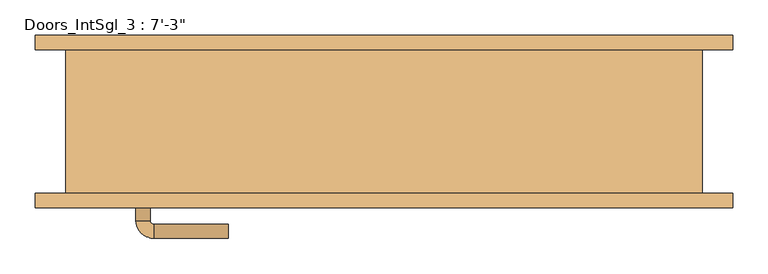
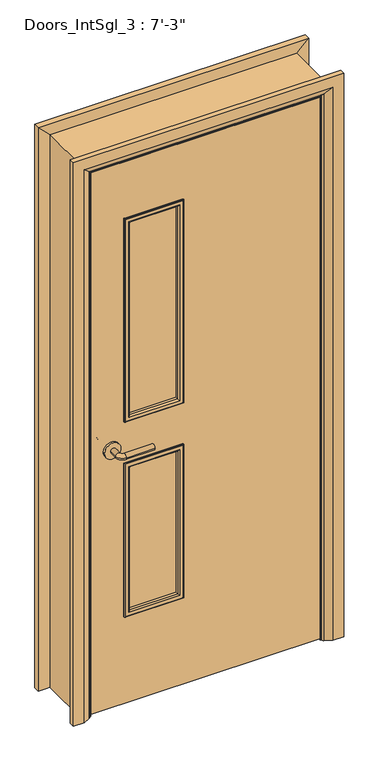
"""IFC4 building model written with IfcOpenShell, lengths in millimetres: door geometry."""

from ifc_helpers import new_model, si_unit, point, frame, frame_2d, origin, place, context, project, spatial, polyline, circle_curve, ellipse_curve, trimmed, segment, composite_curve, outline, extrude, faceted_brep, source, transform, mapped, element, save
from ifc_brep_helpers import plane_surface, cylinder_surface, revolved_surface, advanced_brep


def door_2f4bc105(model_context):
    return source(origin(), model_context, "Body", "SolidModel", [
        advanced_brep(
        [(-350.2, -55.6, 1000.0), (-330.2, -55.6, 1000.0), (-350.2, -25.6, 1000.0), (-330.2, -25.6, 1000.0), (-325.2, -20.6, 1000.0), (-325.2, -0.6, 1000.0), (-220.2, -0.6, 1000.0), (-220.2, -20.6, 1000.0)],
        [
            (0, 1, circle_curve(frame((-340.2, -55.6, 1000.0), z_axis=(0.0, -1.0, 0.0), x_axis=(1.0, 0.0, 0.0)), 10.0)),
            (1, 0, circle_curve(frame((-340.2, -55.6, 1000.0), z_axis=(0.0, -1.0, 0.0), x_axis=(1.0, 0.0, 0.0)), 10.0)),
            (0, 2),
            (2, 3, circle_curve(frame((-340.2, -25.6, 1000.0), z_axis=(0.0, -1.0, 0.0), x_axis=(1.0, 0.0, 0.0)), 10.0)),
            (3, 1),
            (3, 2, circle_curve(frame((-340.2, -25.6, 1000.0), z_axis=(0.0, -1.0, 0.0), x_axis=(1.0, 0.0, 0.0)), 10.0)),
            (4, 3, circle_curve(frame((-325.2, -25.6, 1000.0), z_axis=(0.0, 0.0, 1.0), x_axis=(-1.0, 0.0, 0.0)), 5.0)),
            (2, 5, circle_curve(frame((-325.2, -25.6, 1000.0), z_axis=(0.0, 0.0, -1.0), x_axis=(-1.0, 0.0, 0.0)), 25.0)),
            (5, 4, circle_curve(frame((-325.2, -10.6, 1000.0), z_axis=(-1.0, 0.0, 0.0), x_axis=(0.0, -1.0, 0.0)), 10.0)),
            (4, 5, circle_curve(frame((-325.2, -10.6, 1000.0), z_axis=(-1.0, 0.0, 0.0), x_axis=(0.0, -1.0, 0.0)), 10.0)),
            (6, 7, circle_curve(frame((-220.2, -10.6, 1000.0), z_axis=(1.0, 0.0, 0.0), x_axis=(0.0, -1.0, 0.0)), 10.0)),
            (7, 6, circle_curve(frame((-220.2, -10.6, 1000.0), z_axis=(1.0, 0.0, 0.0), x_axis=(0.0, -1.0, 0.0)), 10.0)),
            (5, 6),
            (7, 4),
        ],
        [
            plane_surface(frame((-340.2, -55.6, 1000.0), z_axis=(0.0, -1.0, 0.0), x_axis=(0.0, 0.0, 1.0))),
            cylinder_surface(frame((-340.2, -55.6, 1000.0), z_axis=(0.0, -1.0, 0.0), x_axis=(1.0, 0.0, 0.0)), 10.0),
            revolved_surface(trimmed(ellipse_curve(frame((-340.2, -25.6, 1000.0), z_axis=(0.0, -1.0, 0.0), x_axis=(1.0, 0.0, 0.0)), 10.0, 10.0), [point((-350.2, -25.6, 1000.0))], [point((-330.2, -25.6, 1000.0))], True, "CARTESIAN"), (-325.2, -25.6, 1000.0), (0.0, 0.0, -1.0)),
            revolved_surface(trimmed(ellipse_curve(frame((-340.2, -25.6, 1000.0), z_axis=(0.0, -1.0, 0.0), x_axis=(1.0, 0.0, 0.0)), 10.0, 10.0), [point((-330.2, -25.6, 1000.0))], [point((-350.2, -25.6, 1000.0))], True, "CARTESIAN"), (-325.2, -25.6, 1000.0), (0.0, 0.0, -1.0)),
            plane_surface(frame((-220.2, -10.6, 1000.0), z_axis=(1.0, 0.0, 0.0), x_axis=(0.0, 0.0, 1.0))),
            cylinder_surface(frame((-325.2, -10.6, 1000.0), z_axis=(-1.0, 0.0, 0.0), x_axis=(0.0, -1.0, 0.0)), 10.0),
        ],
        [
            (0, [[1, 2]]),
            (1, [[-1, 3, 4, 5]]),
            (1, [[-2, -5, 6, -3]]),
            (2, [[7, -4, 8, 9]]),
            (3, [[-8, -6, -7, 10]]),
            (4, [[11, 12]]),
            (5, [[-9, 13, -12, 14]]),
            (5, [[-10, -14, -11, -13]]),
        ],
    ),
        extrude(outline(composite_curve([segment(trimmed(circle_curve(frame_2d((1000.0, -342.7)), 30.0), [point((1000.0, -372.7))], [point((1000.0, -312.7))], False, "CARTESIAN"), True, "CONTINUOUS"), segment(trimmed(circle_curve(frame_2d((1000.0, -342.7)), 30.0), [point((1000.0, -312.7))], [point((1000.0, -372.7))], False, "CARTESIAN"), True, "CONTINUOUS")], self_intersect=False)), frame((0.0, -63.6, 0.0), z_axis=(0.0, 1.0, 0.0), x_axis=(0.0, 0.0, 1.0)), (0.0, 0.0, 1.0), 8.0),
        advanced_brep(
        [(-350.2, -109.6, 1000.0), (-330.2, -109.6, 1000.0), (-330.2, -139.6, 1000.0), (-350.2, -139.6, 1000.0), (-325.2, -144.6, 1000.0), (-325.2, -164.6, 1000.0), (-220.2, -164.6, 1000.0), (-220.2, -144.6, 1000.0)],
        [
            (0, 1, circle_curve(frame((-340.2, -109.6, 1000.0), z_axis=(0.0, 1.0, 0.0), x_axis=(1.0, 0.0, 0.0)), 10.0)),
            (1, 0, circle_curve(frame((-340.2, -109.6, 1000.0), z_axis=(0.0, 1.0, 0.0), x_axis=(1.0, 0.0, 0.0)), 10.0)),
            (1, 2),
            (2, 3, circle_curve(frame((-340.2, -139.6, 1000.0), z_axis=(0.0, 1.0, 0.0), x_axis=(1.0, 0.0, 0.0)), 10.0)),
            (3, 0),
            (3, 2, circle_curve(frame((-340.2, -139.6, 1000.0), z_axis=(0.0, 1.0, 0.0), x_axis=(1.0, 0.0, 0.0)), 10.0)),
            (4, 5, circle_curve(frame((-325.2, -154.6, 1000.0), z_axis=(-1.0, 0.0, 0.0), x_axis=(0.0, 1.0, 0.0)), 10.0)),
            (5, 3, circle_curve(frame((-325.2, -139.6, 1000.0), z_axis=(0.0, 0.0, -1.0), x_axis=(-1.0, 0.0, 0.0)), 25.0)),
            (2, 4, circle_curve(frame((-325.2, -139.6, 1000.0), z_axis=(0.0, 0.0, 1.0), x_axis=(-1.0, 0.0, 0.0)), 5.0)),
            (5, 4, circle_curve(frame((-325.2, -154.6, 1000.0), z_axis=(-1.0, 0.0, 0.0), x_axis=(0.0, 1.0, 0.0)), 10.0)),
            (6, 7, circle_curve(frame((-220.2, -154.6, 1000.0), z_axis=(1.0, 0.0, 0.0), x_axis=(0.0, 1.0, 0.0)), 10.0)),
            (7, 6, circle_curve(frame((-220.2, -154.6, 1000.0), z_axis=(1.0, 0.0, 0.0), x_axis=(0.0, 1.0, 0.0)), 10.0)),
            (4, 7),
            (6, 5),
        ],
        [
            plane_surface(frame((-340.2, -109.6, 1000.0), z_axis=(0.0, 1.0, 0.0), x_axis=(0.0, 0.0, 1.0))),
            cylinder_surface(frame((-340.2, -109.6, 1000.0), z_axis=(0.0, 1.0, 0.0), x_axis=(1.0, 0.0, 0.0)), 10.0),
            revolved_surface(trimmed(ellipse_curve(frame((-340.2, -139.6, 1000.0), z_axis=(0.0, -1.0, 0.0), x_axis=(1.0, 0.0, 0.0)), 10.0, 10.0), [point((-350.2, -139.6, 1000.0))], [point((-330.2, -139.6, 1000.0))], True, "CARTESIAN"), (-325.2, -139.6, 1000.0), (0.0, 0.0, -1.0)),
            revolved_surface(trimmed(ellipse_curve(frame((-340.2, -139.6, 1000.0), z_axis=(0.0, -1.0, 0.0), x_axis=(1.0, 0.0, 0.0)), 10.0, 10.0), [point((-330.2, -139.6, 1000.0))], [point((-350.2, -139.6, 1000.0))], True, "CARTESIAN"), (-325.2, -139.6, 1000.0), (0.0, 0.0, -1.0)),
            plane_surface(frame((-220.2, -154.6, 1000.0), z_axis=(1.0, 0.0, 0.0), x_axis=(0.0, 0.0, 1.0))),
            cylinder_surface(frame((-325.2, -154.6, 1000.0), z_axis=(-1.0, 0.0, 0.0), x_axis=(0.0, 1.0, 0.0)), 10.0),
        ],
        [
            (0, [[1, 2]]),
            (1, [[3, 4, 5, -2]]),
            (1, [[-5, 6, -3, -1]]),
            (2, [[7, 8, -4, 9]]),
            (3, [[10, -9, -6, -8]]),
            (4, [[11, 12]]),
            (5, [[13, -11, 14, -7]]),
            (5, [[-14, -12, -13, -10]]),
        ],
    ),
        extrude(outline(composite_curve([segment(trimmed(circle_curve(frame_2d((1000.0, -342.7)), 30.0), [point((1000.0, -372.7))], [point((1000.0, -312.7))], False, "CARTESIAN"), True, "CONTINUOUS"), segment(trimmed(circle_curve(frame_2d((1000.0, -342.7)), 30.0), [point((1000.0, -312.7))], [point((1000.0, -372.7))], False, "CARTESIAN"), True, "CONTINUOUS")], self_intersect=False)), frame((0.0, -109.6, 0.0), z_axis=(0.0, 1.0, 0.0), x_axis=(0.0, 0.0, 1.0)), (0.0, 0.0, 1.0), 8.0),
        extrude(outline(polyline([(2091.6, -415.2), (8.0, -415.2), (8.0, 415.2), (2091.6, 415.2), (2091.6, -415.2)]), holes=[polyline([(1866.6, -90.2), (1100.0, -90.2), (1100.0, -290.2), (1866.6, -290.2), (1866.6, -90.2)]), polyline([(925.0, -290.2), (925.0, -90.2), (350.0, -90.2), (350.0, -290.2), (925.0, -290.2)])]), frame((0.0, -101.6, 0.0), z_axis=(0.0, 1.0, 0.0), x_axis=(0.0, 0.0, 1.0)), (0.0, 0.0, 1.0), 38.0),
        faceted_brep([(-417.2, -101.6, 0.0), (-449.2, -101.6, 0.0), (-449.2, 101.6, 0.0), (-417.2, 101.6, 0.0), (-417.2, 101.6, 2093.6), (-417.2, -101.6, 2093.6), (-449.2, 101.6, 2125.6), (-449.2, -101.6, 2125.6), (417.2, -101.6, 0.0), (417.2, 101.6, 0.0), (449.2, 101.6, 0.0), (449.2, -101.6, 0.0), (417.2, -101.6, 2093.6), (449.2, -101.6, 2125.6), (449.2, 101.6, 2125.6), (417.2, 101.6, 2093.6)], [[[0, 1, 2, 3]], [[3, 4, 5, 0]], [[2, 6, 4, 3]], [[1, 7, 6, 2]], [[0, 5, 7, 1]], [[8, 9, 10, 11]], [[12, 8, 11, 13]], [[13, 11, 10, 14]], [[14, 10, 9, 15]], [[15, 9, 8, 12]], [[4, 15, 12, 5]], [[6, 14, 15, 4]], [[7, 13, 14, 6]], [[5, 12, 13, 7]]]),
        advanced_brep(
        [(-492.2, 121.6, 0.0), (-452.2, 121.6, 0.0), (-426.2, 107.6, 0.0), (-422.2, 101.6, 0.0), (-492.2, 101.6, 0.0), (-492.2, 101.6, 2168.6), (-492.2, 121.6, 2168.6), (-422.2, 101.6, 2098.6), (-426.2, 107.6, 2102.6), (-452.2, 121.6, 2128.6), (492.2, 121.6, 0.0), (492.2, 101.6, 0.0), (422.2, 101.6, 0.0), (426.2, 107.6, 0.0), (452.2, 121.6, 0.0), (492.2, 121.6, 2168.6), (452.2, 121.6, 2128.6), (426.2, 107.6, 2102.6), (422.2, 101.6, 2098.6), (492.2, 101.6, 2168.6)],
        [
            (0, 1),
            (1, 2),
            (2, 3, circle_curve(frame((-430.2, 100.6, 0.0), z_axis=(0.0, 0.0, -1.0), x_axis=(-1.0, 0.0, 0.0)), 8.0622577)),
            (3, 4),
            (4, 0),
            (4, 5),
            (5, 6),
            (6, 0),
            (3, 7),
            (7, 5),
            (2, 8),
            (8, 7, ellipse_curve(frame((-430.2, 100.6, 2106.6), z_axis=(-0.7071067811865475, 0.0, -0.7071067811865475), x_axis=(0.7071067811865474, 0.0, -0.7071067811865476)), 11.4017543, 8.0622577)),
            (1, 9),
            (9, 8),
            (6, 9),
            (10, 11),
            (11, 12),
            (12, 13, circle_curve(frame((430.2, 100.6, 0.0), z_axis=(0.0, 0.0, -1.0), x_axis=(1.0, 0.0, 0.0)), 8.0622577)),
            (13, 14),
            (14, 10),
            (15, 10),
            (14, 16),
            (16, 15),
            (13, 17),
            (17, 16),
            (12, 18),
            (18, 17, ellipse_curve(frame((430.2, 100.6, 2106.6), z_axis=(0.7071067811865475, 0.0, -0.7071067811865475), x_axis=(0.7071067811865474, 0.0, 0.7071067811865476)), 11.4017543, 8.0622577)),
            (11, 19),
            (19, 18),
            (15, 19),
            (5, 19),
            (15, 6),
            (7, 18),
            (8, 17),
            (9, 16),
        ],
        [
            plane_surface(frame((-422.2, 174.4010989, 0.0), z_axis=(0.0, 0.0, -1.0), x_axis=(1.0, 0.0, 0.0))),
            plane_surface(frame((-492.2, 121.6, 0.0), z_axis=(-1.0, 0.0, 0.0), x_axis=(0.0, 0.0, 1.0))),
            plane_surface(frame((-492.2, 101.6, 0.0), z_axis=(0.0, -1.0, 0.0), x_axis=(0.0, 0.0, 1.0))),
            cylinder_surface(frame((-430.2, 100.6, 0.0), z_axis=(0.0, 0.0, -1.0), x_axis=(-1.0, 0.0, 0.0)), 8.0622577),
            plane_surface(frame((-426.2, 107.6, 0.0), z_axis=(0.4740998230350183, 0.8804710999221749, 0.0), x_axis=(0.0, 0.0, 1.0))),
            plane_surface(frame((-452.2, 121.6, 0.0), z_axis=(0.0, 1.0, 0.0), x_axis=(0.0, 0.0, 1.0))),
            plane_surface(frame((422.2, 174.4010989, 0.0), z_axis=(0.0, 0.0, -1.0), x_axis=(-1.0, 0.0, 0.0))),
            plane_surface(frame((452.2, 121.6, 2128.6), z_axis=(0.0, 1.0, 0.0), x_axis=(0.0, 0.0, -1.0))),
            plane_surface(frame((426.2, 107.6, 2102.6), z_axis=(-0.4740998230350183, 0.8804710999221749, 0.0), x_axis=(0.0, 0.0, -1.0))),
            cylinder_surface(frame((430.2, 100.6, 2098.6), z_axis=(0.0, 0.0, 1.0), x_axis=(1.0, 0.0, 0.0)), 8.0622577),
            plane_surface(frame((492.2, 101.6, 2168.6), z_axis=(0.0, -1.0, 0.0), x_axis=(0.0, 0.0, -1.0))),
            plane_surface(frame((492.2, 121.6, 2168.6), z_axis=(1.0, 0.0, 0.0), x_axis=(0.0, 0.0, -1.0))),
            plane_surface(frame((-492.2, 121.6, 2168.6), z_axis=(0.0, 0.0, 1.0), x_axis=(1.0, 0.0, 0.0))),
            plane_surface(frame((-492.2, 101.6, 2168.6), z_axis=(0.0, -1.0, 0.0), x_axis=(1.0, 0.0, 0.0))),
            cylinder_surface(frame((-422.2, 100.6, 2106.6), z_axis=(-1.0, 0.0, 0.0), x_axis=(0.0, 0.0, 1.0)), 8.0622577),
            plane_surface(frame((-426.2, 107.6, 2102.6), z_axis=(0.0, 0.8804710999221749, -0.4740998230350183), x_axis=(1.0, 0.0, 0.0))),
            plane_surface(frame((-452.2, 121.6, 2128.6), z_axis=(0.0, 1.0, 0.0), x_axis=(1.0, 0.0, 0.0))),
        ],
        [
            (0, [[1, 2, 3, 4, 5]]),
            (1, [[6, 7, 8, -5]]),
            (2, [[9, 10, -6, -4]]),
            (3, [[11, 12, -9, -3]]),
            (4, [[13, 14, -11, -2]]),
            (5, [[-8, 15, -13, -1]]),
            (6, [[16, 17, 18, 19, 20]]),
            (7, [[21, -20, 22, 23]]),
            (8, [[-22, -19, 24, 25]]),
            (9, [[-24, -18, 26, 27]]),
            (10, [[-26, -17, 28, 29]]),
            (11, [[-28, -16, -21, 30]]),
            (12, [[31, -30, 32, -7]]),
            (13, [[33, -29, -31, -10]]),
            (14, [[34, -27, -33, -12]]),
            (15, [[35, -25, -34, -14]]),
            (16, [[-32, -23, -35, -15]]),
        ],
    ),
        extrude(outline(polyline([(0.0, -398.2), (2074.6, -398.2), (2074.6, 398.2), (0.0, 398.2), (0.0, 417.2), (2093.6, 417.2), (2093.6, -417.2), (0.0, -417.2), (0.0, -398.2)])), frame((0.0, -61.6, 0.0), z_axis=(0.0, 1.0, 0.0), x_axis=(0.0, 0.0, 1.0)), (0.0, 0.0, 1.0), 32.0),
        advanced_brep(
        [(492.2, -121.6, 0.0), (452.2, -121.6, 0.0), (426.2, -107.6, 0.0), (422.2, -101.6, 0.0), (492.2, -101.6, 0.0), (492.2, -101.6, 2168.6), (492.2, -121.6, 2168.6), (422.2, -101.6, 2098.6), (-422.2, -101.6, 2098.6), (-422.2, -101.6, 0.0), (-492.2, -101.6, 0.0), (-492.2, -101.6, 2168.6), (426.2, -107.6, 2102.6), (452.2, -121.6, 2128.6), (-492.2, -121.6, 2168.6), (-492.2, -121.6, 0.0), (-452.2, -121.6, 0.0), (-452.2, -121.6, 2128.6), (-426.2, -107.6, 0.0), (-426.2, -107.6, 2102.6)],
        [
            (0, 1),
            (1, 2),
            (2, 3, circle_curve(frame((430.2, -100.6, 0.0), z_axis=(0.0, 0.0, -1.0), x_axis=(1.0, 0.0, 0.0)), 8.0622577)),
            (3, 4),
            (4, 0),
            (4, 5),
            (5, 6),
            (6, 0),
            (3, 7),
            (7, 8),
            (8, 9),
            (9, 10),
            (10, 11),
            (11, 5),
            (2, 12),
            (12, 7, ellipse_curve(frame((430.2, -100.6, 2106.6), z_axis=(0.7071067811865475, 0.0, -0.7071067811865475), x_axis=(-0.7071067811865474, 0.0, -0.7071067811865476)), 11.4017543, 8.0622577)),
            (1, 13),
            (13, 12),
            (6, 14),
            (14, 15),
            (15, 16),
            (16, 17),
            (17, 13),
            (10, 15),
            (14, 11),
            (9, 18, circle_curve(frame((-430.2, -100.6, 0.0), z_axis=(0.0, 0.0, -1.0), x_axis=(-1.0, 0.0, 0.0)), 8.0622577)),
            (18, 16),
            (19, 18),
            (8, 19, ellipse_curve(frame((-430.2, -100.6, 2106.6), z_axis=(-0.7071067811865475, 0.0, -0.7071067811865475), x_axis=(-0.7071067811865474, 0.0, 0.7071067811865476)), 11.4017543, 8.0622577)),
            (19, 17),
            (12, 19),
        ],
        [
            plane_surface(frame((422.2, -101.6, 0.0), z_axis=(0.0, 0.0, -1.0), x_axis=(0.0, 1.0, 0.0))),
            plane_surface(frame((492.2, -121.6, 0.0), z_axis=(1.0, 0.0, 0.0), x_axis=(0.0, 0.0, 1.0))),
            plane_surface(frame((492.2, -101.6, 0.0), z_axis=(0.0, 1.0, 0.0), x_axis=(0.0, 0.0, 1.0))),
            cylinder_surface(frame((430.2, -100.6, 0.0), z_axis=(0.0, 0.0, -1.0), x_axis=(1.0, 0.0, 0.0)), 8.0622577),
            plane_surface(frame((426.2, -107.6, 0.0), z_axis=(-0.4740998230350126, -0.8804710999221779, 0.0), x_axis=(0.0, 0.0, 1.0))),
            plane_surface(frame((452.2, -121.6, 0.0), z_axis=(0.0, -1.0, 0.0), x_axis=(0.0, 0.0, 1.0))),
            plane_surface(frame((-492.2, -121.6, 2168.6), z_axis=(-1.0, 0.0, 0.0), x_axis=(0.0, 0.0, -1.0))),
            plane_surface(frame((-422.2, -101.6, 0.0), z_axis=(0.0, 0.0, -1.0), x_axis=(0.0, 1.0, 0.0))),
            cylinder_surface(frame((-430.2, -100.6, 2098.6), z_axis=(0.0, 0.0, 1.0), x_axis=(-1.0, 0.0, 0.0)), 8.0622577),
            plane_surface(frame((-426.2, -107.6, 2102.6), z_axis=(0.4740998230350183, -0.8804710999221749, 0.0), x_axis=(0.0, 0.0, -1.0))),
            plane_surface(frame((492.2, -121.6, 2168.6), z_axis=(0.0, 0.0, 1.0), x_axis=(-1.0, 0.0, 0.0))),
            cylinder_surface(frame((422.2, -100.6, 2106.6), z_axis=(1.0, 0.0, 0.0), x_axis=(0.0, 0.0, 1.0)), 8.0622577),
            plane_surface(frame((426.2, -107.6, 2102.6), z_axis=(0.0, -0.8804710999221763, -0.4740998230350154), x_axis=(-1.0, 0.0, 0.0))),
        ],
        [
            (0, [[1, 2, 3, 4, 5]]),
            (1, [[6, 7, 8, -5]]),
            (2, [[9, 10, 11, 12, 13, 14, -6, -4]]),
            (3, [[15, 16, -9, -3]]),
            (4, [[17, 18, -15, -2]]),
            (5, [[-8, 19, 20, 21, 22, 23, -17, -1]]),
            (6, [[-13, 24, -20, 25]]),
            (7, [[-24, -12, 26, 27, -21]]),
            (8, [[28, -26, -11, 29]]),
            (9, [[-22, -27, -28, 30]]),
            (10, [[-14, -25, -19, -7]]),
            (11, [[31, -29, -10, -16]]),
            (12, [[-23, -30, -31, -18]]),
        ],
    ),
        advanced_brep(
        [(-82.2, -105.6, 1874.6), (-82.2, -105.6, 1092.0), (-82.2, -101.6, 1092.0), (-82.2, -101.6, 1874.6), (-84.2, -107.6, 1872.6), (-84.2, -107.6, 1094.0), (-102.2, -102.6, 1854.6), (-102.2, -102.6, 1112.0), (-97.2, -107.6, 1107.0), (-97.2, -107.6, 1859.6), (-102.2, -91.6, 1854.6), (-102.2, -91.6, 1112.0), (-90.2, -101.6, 1866.6), (-90.2, -101.6, 1100.0), (-90.2, -91.6, 1100.0), (-90.2, -91.6, 1866.6), (-298.2, -105.6, 1092.0), (-298.2, -101.6, 1092.0), (-296.2, -107.6, 1094.0), (-278.2, -102.6, 1112.0), (-283.2, -107.6, 1107.0), (-278.2, -91.6, 1112.0), (-290.2, -101.6, 1100.0), (-290.2, -91.6, 1100.0), (-298.2, -105.6, 1874.6), (-298.2, -101.6, 1874.6), (-296.2, -107.6, 1872.6), (-278.2, -102.6, 1854.6), (-283.2, -107.6, 1859.6), (-278.2, -91.6, 1854.6), (-290.2, -101.6, 1866.6), (-290.2, -91.6, 1866.6)],
        [
            (0, 1),
            (1, 2),
            (2, 3),
            (3, 0),
            (4, 5),
            (5, 1, ellipse_curve(frame((-84.2, -105.6, 1094.0), z_axis=(0.7071067811865475, 0.0, 0.7071067811865475), x_axis=(-0.7071067811865474, 0.0, 0.7071067811865476)), 2.8284271, 2.0)),
            (0, 4, ellipse_curve(frame((-84.2, -105.6, 1872.6), z_axis=(0.7071067811865475, 0.0, -0.7071067811865475), x_axis=(0.7071067811865474, 0.0, 0.7071067811865476)), 2.8284271, 2.0)),
            (6, 7),
            (7, 8, ellipse_curve(frame((-97.2, -102.6, 1107.0), z_axis=(0.7071067811865475, 0.0, 0.7071067811865475), x_axis=(-0.7071067811865474, 0.0, 0.7071067811865476)), 7.0710678, 5.0)),
            (8, 9),
            (9, 6, ellipse_curve(frame((-97.2, -102.6, 1859.6), z_axis=(0.7071067811865475, 0.0, -0.7071067811865475), x_axis=(0.7071067811865474, 0.0, 0.7071067811865476)), 7.0710678, 5.0)),
            (10, 11),
            (11, 7),
            (6, 10),
            (12, 13),
            (13, 14),
            (14, 15),
            (15, 12),
            (1, 16),
            (16, 17),
            (17, 2),
            (5, 18),
            (18, 16, ellipse_curve(frame((-296.2, -105.6, 1094.0), z_axis=(0.7071067811865475, 0.0, -0.7071067811865475), x_axis=(0.7071067811865476, 0.0, 0.7071067811865474)), 2.8284271, 2.0)),
            (7, 19),
            (19, 20, ellipse_curve(frame((-283.2, -102.6, 1107.0), z_axis=(0.7071067811865475, 0.0, -0.7071067811865475), x_axis=(0.7071067811865476, 0.0, 0.7071067811865474)), 7.0710678, 5.0)),
            (20, 8),
            (11, 21),
            (21, 19),
            (13, 22),
            (22, 23),
            (23, 14),
            (16, 24),
            (24, 25),
            (25, 17),
            (18, 26),
            (26, 24, ellipse_curve(frame((-296.2, -105.6, 1872.6), z_axis=(-0.7071067811865475, 0.0, -0.7071067811865475), x_axis=(0.7071067811865474, 0.0, -0.7071067811865476)), 2.8284271, 2.0)),
            (19, 27),
            (27, 28, ellipse_curve(frame((-283.2, -102.6, 1859.6), z_axis=(-0.7071067811865475, 0.0, -0.7071067811865475), x_axis=(0.7071067811865474, 0.0, -0.7071067811865476)), 7.0710678, 5.0)),
            (28, 20),
            (21, 29),
            (29, 27),
            (22, 30),
            (30, 31),
            (31, 23),
            (24, 0),
            (3, 25),
            (26, 4),
            (28, 9),
            (27, 6),
            (29, 10),
            (31, 15),
            (30, 12),
        ],
        [
            plane_surface(frame((-82.2, -101.6, 1874.6), z_axis=(1.0, 0.0, 0.0), x_axis=(0.0, 0.0, -1.0))),
            cylinder_surface(frame((-84.2, -105.6, 1866.6), z_axis=(0.0, 0.0, 1.0), x_axis=(1.0, 0.0, 0.0)), 2.0),
            cylinder_surface(frame((-97.2, -102.6, 1866.6), z_axis=(0.0, 0.0, 1.0), x_axis=(1.0, 0.0, 0.0)), 5.0),
            plane_surface(frame((-102.2, -102.6, 1854.6), z_axis=(-1.0, 0.0, 0.0), x_axis=(0.0, 0.0, -1.0))),
            plane_surface(frame((-90.2, -91.6, 1866.6), z_axis=(1.0, 0.0, 0.0), x_axis=(0.0, 0.0, -1.0))),
            plane_surface(frame((-82.2, -101.6, 1092.0), z_axis=(0.0, 0.0, -1.0), x_axis=(-1.0, 0.0, 0.0))),
            cylinder_surface(frame((-90.2, -105.6, 1094.0), z_axis=(1.0, 0.0, 0.0), x_axis=(0.0, 0.0, -1.0)), 2.0),
            cylinder_surface(frame((-90.2, -102.6, 1107.0), z_axis=(1.0, 0.0, 0.0), x_axis=(0.0, 0.0, -1.0)), 5.0),
            plane_surface(frame((-102.2, -102.6, 1112.0), z_axis=(0.0, 0.0, 1.0), x_axis=(-1.0, 0.0, 0.0))),
            plane_surface(frame((-90.2, -91.6, 1100.0), z_axis=(0.0, 0.0, -1.0), x_axis=(-1.0, 0.0, 0.0))),
            plane_surface(frame((-298.2, -101.6, 1092.0), z_axis=(-1.0, 0.0, 0.0), x_axis=(0.0, 0.0, 1.0))),
            cylinder_surface(frame((-296.2, -105.6, 1100.0), z_axis=(0.0, 0.0, -1.0), x_axis=(-1.0, 0.0, 0.0)), 2.0),
            cylinder_surface(frame((-283.2, -102.6, 1100.0), z_axis=(0.0, 0.0, -1.0), x_axis=(-1.0, 0.0, 0.0)), 5.0),
            plane_surface(frame((-278.2, -102.6, 1112.0), z_axis=(1.0, 0.0, 0.0), x_axis=(0.0, 0.0, 1.0))),
            plane_surface(frame((-290.2, -91.6, 1100.0), z_axis=(-1.0, 0.0, 0.0), x_axis=(0.0, 0.0, 1.0))),
            plane_surface(frame((-298.2, -101.6, 1874.6), z_axis=(0.0, 0.0, 1.0), x_axis=(1.0, 0.0, 0.0))),
            cylinder_surface(frame((-290.2, -105.6, 1872.6), z_axis=(-1.0, 0.0, 0.0), x_axis=(0.0, 0.0, 1.0)), 2.0),
            plane_surface(frame((-296.2, -107.6, 1872.6), z_axis=(0.0, -1.0, 0.0), x_axis=(1.0, 0.0, 0.0))),
            cylinder_surface(frame((-290.2, -102.6, 1859.6), z_axis=(-1.0, 0.0, 0.0), x_axis=(0.0, 0.0, 1.0)), 5.0),
            plane_surface(frame((-278.2, -102.6, 1854.6), z_axis=(0.0, 0.0, -1.0), x_axis=(1.0, 0.0, 0.0))),
            plane_surface(frame((-278.2, -91.6, 1854.6), z_axis=(0.0, 1.0, 0.0), x_axis=(1.0, 0.0, 0.0))),
            plane_surface(frame((-290.2, -91.6, 1866.6), z_axis=(0.0, 0.0, 1.0), x_axis=(1.0, 0.0, 0.0))),
            plane_surface(frame((-290.2, -101.6, 1866.6), z_axis=(0.0, 1.0, 0.0), x_axis=(1.0, 0.0, 0.0))),
        ],
        [
            (0, [[1, 2, 3, 4]]),
            (1, [[5, 6, -1, 7]]),
            (2, [[8, 9, 10, 11]]),
            (3, [[12, 13, -8, 14]]),
            (4, [[15, 16, 17, 18]]),
            (5, [[19, 20, 21, -2]]),
            (6, [[22, 23, -19, -6]]),
            (7, [[24, 25, 26, -9]]),
            (8, [[27, 28, -24, -13]]),
            (9, [[29, 30, 31, -16]]),
            (10, [[32, 33, 34, -20]]),
            (11, [[35, 36, -32, -23]]),
            (12, [[37, 38, 39, -25]]),
            (13, [[40, 41, -37, -28]]),
            (14, [[42, 43, 44, -30]]),
            (15, [[45, -4, 46, -33]]),
            (16, [[47, -7, -45, -36]]),
            (17, [[-5, -47, -35, -22], [-10, -26, -39, 48]]),
            (18, [[49, -11, -48, -38]]),
            (19, [[50, -14, -49, -41]]),
            (20, [[-17, -31, -44, 51], [-12, -50, -40, -27]]),
            (21, [[52, -18, -51, -43]]),
            (22, [[-3, -21, -34, -46], [-15, -52, -42, -29]]),
        ],
    ),
        advanced_brep(
        [(-90.2, -73.6, 1866.6), (-90.2, -73.6, 1100.0), (-90.2, -63.6, 1100.0), (-90.2, -63.6, 1866.6), (-102.2, -62.6, 1854.6), (-102.2, -62.6, 1112.0), (-102.2, -73.6, 1112.0), (-102.2, -73.6, 1854.6), (-97.2, -57.6, 1859.6), (-97.2, -57.6, 1107.0), (-82.2, -59.6, 1874.6), (-82.2, -59.6, 1092.0), (-84.2, -57.6, 1094.0), (-84.2, -57.6, 1872.6), (-82.2, -63.6, 1874.6), (-82.2, -63.6, 1092.0), (-290.2, -73.6, 1100.0), (-290.2, -63.6, 1100.0), (-278.2, -62.6, 1112.0), (-278.2, -73.6, 1112.0), (-283.2, -57.6, 1107.0), (-298.2, -59.6, 1092.0), (-296.2, -57.6, 1094.0), (-298.2, -63.6, 1092.0), (-290.2, -73.6, 1866.6), (-290.2, -63.6, 1866.6), (-278.2, -62.6, 1854.6), (-278.2, -73.6, 1854.6), (-283.2, -57.6, 1859.6), (-298.2, -59.6, 1874.6), (-296.2, -57.6, 1872.6), (-298.2, -63.6, 1874.6)],
        [
            (0, 1),
            (1, 2),
            (2, 3),
            (3, 0),
            (4, 5),
            (5, 6),
            (6, 7),
            (7, 4),
            (8, 9),
            (9, 5, ellipse_curve(frame((-97.2, -62.6, 1107.0), z_axis=(0.7071067811865475, 0.0, 0.7071067811865475), x_axis=(-0.7071067811865474, 0.0, 0.7071067811865476)), 7.0710678, 5.0)),
            (4, 8, ellipse_curve(frame((-97.2, -62.6, 1859.6), z_axis=(0.7071067811865475, 0.0, -0.7071067811865475), x_axis=(0.7071067811865474, 0.0, 0.7071067811865476)), 7.0710678, 5.0)),
            (10, 11),
            (11, 12, ellipse_curve(frame((-84.2, -59.6, 1094.0), z_axis=(0.7071067811865475, 0.0, 0.7071067811865475), x_axis=(-0.7071067811865474, 0.0, 0.7071067811865476)), 2.8284271, 2.0)),
            (12, 13),
            (13, 10, ellipse_curve(frame((-84.2, -59.6, 1872.6), z_axis=(0.7071067811865475, 0.0, -0.7071067811865475), x_axis=(0.7071067811865474, 0.0, 0.7071067811865476)), 2.8284271, 2.0)),
            (14, 15),
            (15, 11),
            (10, 14),
            (1, 16),
            (16, 17),
            (17, 2),
            (5, 18),
            (18, 19),
            (19, 6),
            (9, 20),
            (20, 18, ellipse_curve(frame((-283.2, -62.6, 1107.0), z_axis=(0.7071067811865475, 0.0, -0.7071067811865475), x_axis=(0.7071067811865476, 0.0, 0.7071067811865474)), 7.0710678, 5.0)),
            (11, 21),
            (21, 22, ellipse_curve(frame((-296.2, -59.6, 1094.0), z_axis=(0.7071067811865475, 0.0, -0.7071067811865475), x_axis=(0.7071067811865476, 0.0, 0.7071067811865474)), 2.8284271, 2.0)),
            (22, 12),
            (15, 23),
            (23, 21),
            (16, 24),
            (24, 25),
            (25, 17),
            (18, 26),
            (26, 27),
            (27, 19),
            (20, 28),
            (28, 26, ellipse_curve(frame((-283.2, -62.6, 1859.6), z_axis=(-0.7071067811865475, 0.0, -0.7071067811865475), x_axis=(0.7071067811865474, 0.0, -0.7071067811865476)), 7.0710678, 5.0)),
            (21, 29),
            (29, 30, ellipse_curve(frame((-296.2, -59.6, 1872.6), z_axis=(-0.7071067811865475, 0.0, -0.7071067811865475), x_axis=(0.7071067811865474, 0.0, -0.7071067811865476)), 2.8284271, 2.0)),
            (30, 22),
            (23, 31),
            (31, 29),
            (14, 31),
            (25, 3),
            (24, 0),
            (27, 7),
            (26, 4),
            (28, 8),
            (30, 13),
            (29, 10),
        ],
        [
            plane_surface(frame((-90.2, -63.6, 1866.6), z_axis=(1.0, 0.0, 0.0), x_axis=(0.0, 0.0, -1.0))),
            plane_surface(frame((-102.2, -73.6, 1854.6), z_axis=(-1.0, 0.0, 0.0), x_axis=(0.0, 0.0, -1.0))),
            cylinder_surface(frame((-97.2, -62.6, 1866.6), z_axis=(0.0, 0.0, 1.0), x_axis=(1.0, 0.0, 0.0)), 5.0),
            cylinder_surface(frame((-84.2, -59.6, 1866.6), z_axis=(0.0, 0.0, 1.0), x_axis=(1.0, 0.0, 0.0)), 2.0),
            plane_surface(frame((-82.2, -59.6, 1874.6), z_axis=(1.0, 0.0, 0.0), x_axis=(0.0, 0.0, -1.0))),
            plane_surface(frame((-90.2, -63.6, 1100.0), z_axis=(0.0, 0.0, -1.0), x_axis=(-1.0, 0.0, 0.0))),
            plane_surface(frame((-102.2, -73.6, 1112.0), z_axis=(0.0, 0.0, 1.0), x_axis=(-1.0, 0.0, 0.0))),
            cylinder_surface(frame((-90.2, -62.6, 1107.0), z_axis=(1.0, 0.0, 0.0), x_axis=(0.0, 0.0, -1.0)), 5.0),
            cylinder_surface(frame((-90.2, -59.6, 1094.0), z_axis=(1.0, 0.0, 0.0), x_axis=(0.0, 0.0, -1.0)), 2.0),
            plane_surface(frame((-82.2, -59.6, 1092.0), z_axis=(0.0, 0.0, -1.0), x_axis=(-1.0, 0.0, 0.0))),
            plane_surface(frame((-290.2, -63.6, 1100.0), z_axis=(-1.0, 0.0, 0.0), x_axis=(0.0, 0.0, 1.0))),
            plane_surface(frame((-278.2, -73.6, 1112.0), z_axis=(1.0, 0.0, 0.0), x_axis=(0.0, 0.0, 1.0))),
            cylinder_surface(frame((-283.2, -62.6, 1100.0), z_axis=(0.0, 0.0, -1.0), x_axis=(-1.0, 0.0, 0.0)), 5.0),
            cylinder_surface(frame((-296.2, -59.6, 1100.0), z_axis=(0.0, 0.0, -1.0), x_axis=(-1.0, 0.0, 0.0)), 2.0),
            plane_surface(frame((-298.2, -59.6, 1092.0), z_axis=(-1.0, 0.0, 0.0), x_axis=(0.0, 0.0, 1.0))),
            plane_surface(frame((-298.2, -63.6, 1874.6), z_axis=(0.0, -1.0, 0.0), x_axis=(1.0, 0.0, 0.0))),
            plane_surface(frame((-290.2, -63.6, 1866.6), z_axis=(0.0, 0.0, 1.0), x_axis=(1.0, 0.0, 0.0))),
            plane_surface(frame((-290.2, -73.6, 1866.6), z_axis=(0.0, -1.0, 0.0), x_axis=(1.0, 0.0, 0.0))),
            plane_surface(frame((-278.2, -73.6, 1854.6), z_axis=(0.0, 0.0, -1.0), x_axis=(1.0, 0.0, 0.0))),
            cylinder_surface(frame((-290.2, -62.6, 1859.6), z_axis=(-1.0, 0.0, 0.0), x_axis=(0.0, 0.0, 1.0)), 5.0),
            plane_surface(frame((-283.2, -57.6, 1859.6), z_axis=(0.0, 1.0, 0.0), x_axis=(1.0, 0.0, 0.0))),
            cylinder_surface(frame((-290.2, -59.6, 1872.6), z_axis=(-1.0, 0.0, 0.0), x_axis=(0.0, 0.0, 1.0)), 2.0),
            plane_surface(frame((-298.2, -59.6, 1874.6), z_axis=(0.0, 0.0, 1.0), x_axis=(1.0, 0.0, 0.0))),
        ],
        [
            (0, [[1, 2, 3, 4]]),
            (1, [[5, 6, 7, 8]]),
            (2, [[9, 10, -5, 11]]),
            (3, [[12, 13, 14, 15]]),
            (4, [[16, 17, -12, 18]]),
            (5, [[19, 20, 21, -2]]),
            (6, [[22, 23, 24, -6]]),
            (7, [[25, 26, -22, -10]]),
            (8, [[27, 28, 29, -13]]),
            (9, [[30, 31, -27, -17]]),
            (10, [[32, 33, 34, -20]]),
            (11, [[35, 36, 37, -23]]),
            (12, [[38, 39, -35, -26]]),
            (13, [[40, 41, 42, -28]]),
            (14, [[43, 44, -40, -31]]),
            (15, [[-16, 45, -43, -30], [-3, -21, -34, 46]]),
            (16, [[47, -4, -46, -33]]),
            (17, [[-1, -47, -32, -19], [-7, -24, -37, 48]]),
            (18, [[49, -8, -48, -36]]),
            (19, [[50, -11, -49, -39]]),
            (20, [[-14, -29, -42, 51], [-9, -50, -38, -25]]),
            (21, [[52, -15, -51, -41]]),
            (22, [[-45, -18, -52, -44]]),
        ],
    ),
        extrude(outline(polyline([(-290.2, -91.6), (-290.2, -73.6), (-90.2, -73.6), (-90.2, -91.6), (-290.2, -91.6)])), frame((0.0, 0.0, 1100.0), z_axis=(0.0, 0.0, 1.0), x_axis=(1.0, 0.0, 0.0)), (0.0, 0.0, 1.0), 766.6),
        extrude(outline(polyline([(-290.2, -91.6), (-290.2, -73.6), (-90.2, -73.6), (-90.2, -91.6), (-290.2, -91.6)])), frame((0.0, 0.0, 350.0), z_axis=(0.0, 0.0, 1.0), x_axis=(1.0, 0.0, 0.0)), (0.0, 0.0, 1.0), 575.0),
        advanced_brep(
        [(-290.2, -91.6, 925.0), (-290.2, -91.6, 350.0), (-290.2, -101.6, 350.0), (-290.2, -101.6, 925.0), (-278.2, -102.6, 913.0), (-278.2, -102.6, 362.0), (-278.2, -91.6, 362.0), (-278.2, -91.6, 913.0), (-283.2, -107.6, 918.0), (-283.2, -107.6, 357.0), (-298.2, -105.6, 933.0), (-298.2, -105.6, 342.0), (-296.2, -107.6, 344.0), (-296.2, -107.6, 931.0), (-298.2, -101.6, 933.0), (-298.2, -101.6, 342.0), (-90.2, -91.6, 350.0), (-90.2, -101.6, 350.0), (-102.2, -102.6, 362.0), (-102.2, -91.6, 362.0), (-97.2, -107.6, 357.0), (-82.2, -105.6, 342.0), (-84.2, -107.6, 344.0), (-82.2, -101.6, 342.0), (-90.2, -91.6, 925.0), (-90.2, -101.6, 925.0), (-102.2, -102.6, 913.0), (-102.2, -91.6, 913.0), (-97.2, -107.6, 918.0), (-82.2, -105.6, 933.0), (-84.2, -107.6, 931.0), (-82.2, -101.6, 933.0)],
        [
            (0, 1),
            (1, 2),
            (2, 3),
            (3, 0),
            (4, 5),
            (5, 6),
            (6, 7),
            (7, 4),
            (8, 9),
            (9, 5, ellipse_curve(frame((-283.2, -102.6, 357.0), z_axis=(-0.7071067811865475, 0.0, 0.7071067811865475), x_axis=(0.7071067811865474, 0.0, 0.7071067811865476)), 7.0710678, 5.0)),
            (4, 8, ellipse_curve(frame((-283.2, -102.6, 918.0), z_axis=(-0.7071067811865475, 0.0, -0.7071067811865475), x_axis=(-0.7071067811865474, 0.0, 0.7071067811865476)), 7.0710678, 5.0)),
            (10, 11),
            (11, 12, ellipse_curve(frame((-296.2, -105.6, 344.0), z_axis=(-0.7071067811865475, 0.0, 0.7071067811865475), x_axis=(0.7071067811865474, 0.0, 0.7071067811865476)), 2.8284271, 2.0)),
            (12, 13),
            (13, 10, ellipse_curve(frame((-296.2, -105.6, 931.0), z_axis=(-0.7071067811865475, 0.0, -0.7071067811865475), x_axis=(-0.7071067811865474, 0.0, 0.7071067811865476)), 2.8284271, 2.0)),
            (14, 15),
            (15, 11),
            (10, 14),
            (1, 16),
            (16, 17),
            (17, 2),
            (5, 18),
            (18, 19),
            (19, 6),
            (9, 20),
            (20, 18, ellipse_curve(frame((-97.2, -102.6, 357.0), z_axis=(-0.7071067811865475, 0.0, -0.7071067811865475), x_axis=(-0.7071067811865476, 0.0, 0.7071067811865474)), 7.0710678, 5.0)),
            (11, 21),
            (21, 22, ellipse_curve(frame((-84.2, -105.6, 344.0), z_axis=(-0.7071067811865475, 0.0, -0.7071067811865475), x_axis=(-0.7071067811865476, 0.0, 0.7071067811865474)), 2.8284271, 2.0)),
            (22, 12),
            (15, 23),
            (23, 21),
            (16, 24),
            (24, 25),
            (25, 17),
            (18, 26),
            (26, 27),
            (27, 19),
            (20, 28),
            (28, 26, ellipse_curve(frame((-97.2, -102.6, 918.0), z_axis=(0.7071067811865475, 0.0, -0.7071067811865475), x_axis=(-0.7071067811865474, 0.0, -0.7071067811865476)), 7.0710678, 5.0)),
            (21, 29),
            (29, 30, ellipse_curve(frame((-84.2, -105.6, 931.0), z_axis=(0.7071067811865475, 0.0, -0.7071067811865475), x_axis=(-0.7071067811865474, 0.0, -0.7071067811865476)), 2.8284271, 2.0)),
            (30, 22),
            (23, 31),
            (31, 29),
            (14, 31),
            (25, 3),
            (24, 0),
            (27, 7),
            (26, 4),
            (28, 8),
            (30, 13),
            (29, 10),
        ],
        [
            plane_surface(frame((-290.2, -101.6, 925.0), z_axis=(-1.0, 0.0, 0.0), x_axis=(0.0, 0.0, -1.0))),
            plane_surface(frame((-278.2, -91.6, 913.0), z_axis=(1.0, 0.0, 0.0), x_axis=(0.0, 0.0, -1.0))),
            cylinder_surface(frame((-283.2, -102.6, 925.0), z_axis=(0.0, 0.0, 1.0), x_axis=(-1.0, 0.0, 0.0)), 5.0),
            cylinder_surface(frame((-296.2, -105.6, 925.0), z_axis=(0.0, 0.0, 1.0), x_axis=(-1.0, 0.0, 0.0)), 2.0),
            plane_surface(frame((-298.2, -105.6, 933.0), z_axis=(-1.0, 0.0, 0.0), x_axis=(0.0, 0.0, -1.0))),
            plane_surface(frame((-290.2, -101.6, 350.0), z_axis=(0.0, 0.0, -1.0), x_axis=(1.0, 0.0, 0.0))),
            plane_surface(frame((-278.2, -91.6, 362.0), z_axis=(0.0, 0.0, 1.0), x_axis=(1.0, 0.0, 0.0))),
            cylinder_surface(frame((-290.2, -102.6, 357.0), z_axis=(-1.0, 0.0, 0.0), x_axis=(0.0, 0.0, -1.0)), 5.0),
            cylinder_surface(frame((-290.2, -105.6, 344.0), z_axis=(-1.0, 0.0, 0.0), x_axis=(0.0, 0.0, -1.0)), 2.0),
            plane_surface(frame((-298.2, -105.6, 342.0), z_axis=(0.0, 0.0, -1.0), x_axis=(1.0, 0.0, 0.0))),
            plane_surface(frame((-90.2, -101.6, 350.0), z_axis=(1.0, 0.0, 0.0), x_axis=(0.0, 0.0, 1.0))),
            plane_surface(frame((-102.2, -91.6, 362.0), z_axis=(-1.0, 0.0, 0.0), x_axis=(0.0, 0.0, 1.0))),
            cylinder_surface(frame((-97.2, -102.6, 350.0), z_axis=(0.0, 0.0, -1.0), x_axis=(1.0, 0.0, 0.0)), 5.0),
            cylinder_surface(frame((-84.2, -105.6, 350.0), z_axis=(0.0, 0.0, -1.0), x_axis=(1.0, 0.0, 0.0)), 2.0),
            plane_surface(frame((-82.2, -105.6, 342.0), z_axis=(1.0, 0.0, 0.0), x_axis=(0.0, 0.0, 1.0))),
            plane_surface(frame((-82.2, -101.6, 933.0), z_axis=(0.0, 1.0, 0.0), x_axis=(-1.0, 0.0, 0.0))),
            plane_surface(frame((-90.2, -101.6, 925.0), z_axis=(0.0, 0.0, 1.0), x_axis=(-1.0, 0.0, 0.0))),
            plane_surface(frame((-90.2, -91.6, 925.0), z_axis=(0.0, 1.0, 0.0), x_axis=(-1.0, 0.0, 0.0))),
            plane_surface(frame((-102.2, -91.6, 913.0), z_axis=(0.0, 0.0, -1.0), x_axis=(-1.0, 0.0, 0.0))),
            cylinder_surface(frame((-90.2, -102.6, 918.0), z_axis=(1.0, 0.0, 0.0), x_axis=(0.0, 0.0, 1.0)), 5.0),
            plane_surface(frame((-97.2, -107.6, 918.0), z_axis=(0.0, -1.0, 0.0), x_axis=(-1.0, 0.0, 0.0))),
            cylinder_surface(frame((-90.2, -105.6, 931.0), z_axis=(1.0, 0.0, 0.0), x_axis=(0.0, 0.0, 1.0)), 2.0),
            plane_surface(frame((-82.2, -105.6, 933.0), z_axis=(0.0, 0.0, 1.0), x_axis=(-1.0, 0.0, 0.0))),
        ],
        [
            (0, [[1, 2, 3, 4]]),
            (1, [[5, 6, 7, 8]]),
            (2, [[9, 10, -5, 11]]),
            (3, [[12, 13, 14, 15]]),
            (4, [[16, 17, -12, 18]]),
            (5, [[19, 20, 21, -2]]),
            (6, [[22, 23, 24, -6]]),
            (7, [[25, 26, -22, -10]]),
            (8, [[27, 28, 29, -13]]),
            (9, [[30, 31, -27, -17]]),
            (10, [[32, 33, 34, -20]]),
            (11, [[35, 36, 37, -23]]),
            (12, [[38, 39, -35, -26]]),
            (13, [[40, 41, 42, -28]]),
            (14, [[43, 44, -40, -31]]),
            (15, [[-16, 45, -43, -30], [-3, -21, -34, 46]]),
            (16, [[47, -4, -46, -33]]),
            (17, [[-1, -47, -32, -19], [-7, -24, -37, 48]]),
            (18, [[49, -8, -48, -36]]),
            (19, [[50, -11, -49, -39]]),
            (20, [[-14, -29, -42, 51], [-9, -50, -38, -25]]),
            (21, [[52, -15, -51, -41]]),
            (22, [[-45, -18, -52, -44]]),
        ],
    ),
        advanced_brep(
        [(-90.2, -73.6, 925.0), (-90.2, -73.6, 350.0), (-90.2, -63.6, 350.0), (-90.2, -63.6, 925.0), (-102.2, -62.6, 913.0), (-102.2, -62.6, 362.0), (-102.2, -73.6, 362.0), (-102.2, -73.6, 913.0), (-97.2, -57.6, 918.0), (-97.2, -57.6, 357.0), (-82.2, -59.6, 933.0), (-82.2, -59.6, 342.0), (-84.2, -57.6, 344.0), (-84.2, -57.6, 931.0), (-82.2, -63.6, 933.0), (-82.2, -63.6, 342.0), (-290.2, -73.6, 350.0), (-290.2, -63.6, 350.0), (-278.2, -62.6, 362.0), (-278.2, -73.6, 362.0), (-283.2, -57.6, 357.0), (-298.2, -59.6, 342.0), (-296.2, -57.6, 344.0), (-298.2, -63.6, 342.0), (-290.2, -73.6, 925.0), (-290.2, -63.6, 925.0), (-278.2, -62.6, 913.0), (-278.2, -73.6, 913.0), (-283.2, -57.6, 918.0), (-298.2, -59.6, 933.0), (-296.2, -57.6, 931.0), (-298.2, -63.6, 933.0)],
        [
            (0, 1),
            (1, 2),
            (2, 3),
            (3, 0),
            (4, 5),
            (5, 6),
            (6, 7),
            (7, 4),
            (8, 9),
            (9, 5, ellipse_curve(frame((-97.2, -62.6, 357.0), z_axis=(0.7071067811865475, 0.0, 0.7071067811865475), x_axis=(-0.7071067811865474, 0.0, 0.7071067811865476)), 7.0710678, 5.0)),
            (4, 8, ellipse_curve(frame((-97.2, -62.6, 918.0), z_axis=(0.7071067811865475, 0.0, -0.7071067811865475), x_axis=(0.7071067811865474, 0.0, 0.7071067811865476)), 7.0710678, 5.0)),
            (10, 11),
            (11, 12, ellipse_curve(frame((-84.2, -59.6, 344.0), z_axis=(0.7071067811865475, 0.0, 0.7071067811865475), x_axis=(-0.7071067811865474, 0.0, 0.7071067811865476)), 2.8284271, 2.0)),
            (12, 13),
            (13, 10, ellipse_curve(frame((-84.2, -59.6, 931.0), z_axis=(0.7071067811865475, 0.0, -0.7071067811865475), x_axis=(0.7071067811865474, 0.0, 0.7071067811865476)), 2.8284271, 2.0)),
            (14, 15),
            (15, 11),
            (10, 14),
            (1, 16),
            (16, 17),
            (17, 2),
            (5, 18),
            (18, 19),
            (19, 6),
            (9, 20),
            (20, 18, ellipse_curve(frame((-283.2, -62.6, 357.0), z_axis=(0.7071067811865475, 0.0, -0.7071067811865475), x_axis=(0.7071067811865476, 0.0, 0.7071067811865474)), 7.0710678, 5.0)),
            (11, 21),
            (21, 22, ellipse_curve(frame((-296.2, -59.6, 344.0), z_axis=(0.7071067811865475, 0.0, -0.7071067811865475), x_axis=(0.7071067811865476, 0.0, 0.7071067811865474)), 2.8284271, 2.0)),
            (22, 12),
            (15, 23),
            (23, 21),
            (16, 24),
            (24, 25),
            (25, 17),
            (18, 26),
            (26, 27),
            (27, 19),
            (20, 28),
            (28, 26, ellipse_curve(frame((-283.2, -62.6, 918.0), z_axis=(-0.7071067811865475, 0.0, -0.7071067811865475), x_axis=(0.7071067811865474, 0.0, -0.7071067811865476)), 7.0710678, 5.0)),
            (21, 29),
            (29, 30, ellipse_curve(frame((-296.2, -59.6, 931.0), z_axis=(-0.7071067811865475, 0.0, -0.7071067811865475), x_axis=(0.7071067811865474, 0.0, -0.7071067811865476)), 2.8284271, 2.0)),
            (30, 22),
            (23, 31),
            (31, 29),
            (14, 31),
            (25, 3),
            (24, 0),
            (27, 7),
            (26, 4),
            (28, 8),
            (30, 13),
            (29, 10),
        ],
        [
            plane_surface(frame((-90.2, -63.6, 925.0), z_axis=(1.0, 0.0, 0.0), x_axis=(0.0, 0.0, -1.0))),
            plane_surface(frame((-102.2, -73.6, 913.0), z_axis=(-1.0, 0.0, 0.0), x_axis=(0.0, 0.0, -1.0))),
            cylinder_surface(frame((-97.2, -62.6, 925.0), z_axis=(0.0, 0.0, 1.0), x_axis=(1.0, 0.0, 0.0)), 5.0),
            cylinder_surface(frame((-84.2, -59.6, 925.0), z_axis=(0.0, 0.0, 1.0), x_axis=(1.0, 0.0, 0.0)), 2.0),
            plane_surface(frame((-82.2, -59.6, 933.0), z_axis=(1.0, 0.0, 0.0), x_axis=(0.0, 0.0, -1.0))),
            plane_surface(frame((-90.2, -63.6, 350.0), z_axis=(0.0, 0.0, -1.0), x_axis=(-1.0, 0.0, 0.0))),
            plane_surface(frame((-102.2, -73.6, 362.0), z_axis=(0.0, 0.0, 1.0), x_axis=(-1.0, 0.0, 0.0))),
            cylinder_surface(frame((-90.2, -62.6, 357.0), z_axis=(1.0, 0.0, 0.0), x_axis=(0.0, 0.0, -1.0)), 5.0),
            cylinder_surface(frame((-90.2, -59.6, 344.0), z_axis=(1.0, 0.0, 0.0), x_axis=(0.0, 0.0, -1.0)), 2.0),
            plane_surface(frame((-82.2, -59.6, 342.0), z_axis=(0.0, 0.0, -1.0), x_axis=(-1.0, 0.0, 0.0))),
            plane_surface(frame((-290.2, -63.6, 350.0), z_axis=(-1.0, 0.0, 0.0), x_axis=(0.0, 0.0, 1.0))),
            plane_surface(frame((-278.2, -73.6, 362.0), z_axis=(1.0, 0.0, 0.0), x_axis=(0.0, 0.0, 1.0))),
            cylinder_surface(frame((-283.2, -62.6, 350.0), z_axis=(0.0, 0.0, -1.0), x_axis=(-1.0, 0.0, 0.0)), 5.0),
            cylinder_surface(frame((-296.2, -59.6, 350.0), z_axis=(0.0, 0.0, -1.0), x_axis=(-1.0, 0.0, 0.0)), 2.0),
            plane_surface(frame((-298.2, -59.6, 342.0), z_axis=(-1.0, 0.0, 0.0), x_axis=(0.0, 0.0, 1.0))),
            plane_surface(frame((-298.2, -63.6, 933.0), z_axis=(0.0, -1.0, 0.0), x_axis=(1.0, 0.0, 0.0))),
            plane_surface(frame((-290.2, -63.6, 925.0), z_axis=(0.0, 0.0, 1.0), x_axis=(1.0, 0.0, 0.0))),
            plane_surface(frame((-290.2, -73.6, 925.0), z_axis=(0.0, -1.0, 0.0), x_axis=(1.0, 0.0, 0.0))),
            plane_surface(frame((-278.2, -73.6, 913.0), z_axis=(0.0, 0.0, -1.0), x_axis=(1.0, 0.0, 0.0))),
            cylinder_surface(frame((-290.2, -62.6, 918.0), z_axis=(-1.0, 0.0, 0.0), x_axis=(0.0, 0.0, 1.0)), 5.0),
            plane_surface(frame((-283.2, -57.6, 918.0), z_axis=(0.0, 1.0, 0.0), x_axis=(1.0, 0.0, 0.0))),
            cylinder_surface(frame((-290.2, -59.6, 931.0), z_axis=(-1.0, 0.0, 0.0), x_axis=(0.0, 0.0, 1.0)), 2.0),
            plane_surface(frame((-298.2, -59.6, 933.0), z_axis=(0.0, 0.0, 1.0), x_axis=(1.0, 0.0, 0.0))),
        ],
        [
            (0, [[1, 2, 3, 4]]),
            (1, [[5, 6, 7, 8]]),
            (2, [[9, 10, -5, 11]]),
            (3, [[12, 13, 14, 15]]),
            (4, [[16, 17, -12, 18]]),
            (5, [[19, 20, 21, -2]]),
            (6, [[22, 23, 24, -6]]),
            (7, [[25, 26, -22, -10]]),
            (8, [[27, 28, 29, -13]]),
            (9, [[30, 31, -27, -17]]),
            (10, [[32, 33, 34, -20]]),
            (11, [[35, 36, 37, -23]]),
            (12, [[38, 39, -35, -26]]),
            (13, [[40, 41, 42, -28]]),
            (14, [[43, 44, -40, -31]]),
            (15, [[-16, 45, -43, -30], [-3, -21, -34, 46]]),
            (16, [[47, -4, -46, -33]]),
            (17, [[-1, -47, -32, -19], [-7, -24, -37, 48]]),
            (18, [[49, -8, -48, -36]]),
            (19, [[50, -11, -49, -39]]),
            (20, [[-14, -29, -42, 51], [-9, -50, -38, -25]]),
            (21, [[52, -15, -51, -41]]),
            (22, [[-45, -18, -52, -44]]),
        ],
    ),
    ])


if __name__ == "__main__":
    model = new_model("IFC4")
    model_context = context("Model", 3, world=origin())
    ifc_project = project(units=[si_unit("LENGTHUNIT", "METRE", prefix="MILLI")], contexts=[model_context])
    site = spatial("IfcSite", under=ifc_project)
    building = spatial("IfcBuilding", under=site)
    placement = place(None, origin())
    door_shape = door_2f4bc105(model_context)
    element("IfcDoor", 1, ObjectType="Doors_IntSgl_3 : 7'-3\"", at=placement, inside=building, context=model_context, shape_type="MappedRepresentation", body=[
        mapped(door_shape, transform((0.0, 0.0, 0.0), x_axis=(1.0, 0.0, 0.0), y_axis=(0.0, 1.0, 0.0), z_axis=(0.0, 0.0, 1.0))),
    ])
    save(model, "model.ifc")

# Revit data of these elements
# Type "Doors_IntSgl_3 : 7'-3\""
#   Type Mark = "14"
#   Type Comments = "Internal Single"
#   Operation = "SingleSwingRight"
#   Construction Type Id = "SGL"
#   Manufacturer = "Revit"
#   Keynote = "L20"
#   Description = "Internal Single Door"
#   Analytic Construction = "Large single-glazed windows"
#   Visual Light Transmittance = 0.9
#   VisionPanel Width = 0' - 7.87402"
#   UnderCut = 0' - 0.31496"
#   Tolerance = 0' - 0.07874"
#   Structural Tolerance = 0' - 0.31496"
#   StopDepth = 0' - 1.25984"
#   Stop Thickness = 0' - 0.74803"
#   Stile Top of Lock Rail = 3' - 7.30709"
#   Stile Top Rail = 0' - 8.85827"
#   Stile Shutting = 0' - 4.92126"
#   Stile Lock Rail = 0' - 6.88976"
#   Stile Bottom Rail = 1' - 1.77953"
#   Solar Heat Gain Coefficient = 0.86
#   Rough Width = 3' - 0"
#   Rough Height = 7' - 0"
#   Heat Transfer Coefficient (U) = 0.979472 BTU/(h·ft²·°F)
#   Handle Z Distance = 3' - 3.37008"
#   Handle X Distance = 0' - 2.95276"
#   Frame Thickness = 0' - 1.25984"
#   Door Panel Width = 2' - 8.69291"
#   Door Panel Thickness = 0' - 1.49606"
#   Door Panel Offset = 0' - 0"
#   Height = 7' - 0"
#   Width = 3' - 0"
#   Door Panel Height = 6' - 10.0315"
#   Architrave Setback = 0' - 0.19685"
#   Vis - Ironmongery = yes
#   Define Thermal Properties by = 1
#   Material Ironmongery = Door - Handle
#   Material Glass = Door - Glazing
#   Material Frame = Door - Frame/Mullion
#   Material Door = Door - Panel
#   Material Beading = Door - Panel
#   Material Architrave = Door - Architrave
#   Function = (empty or 0)
#   Wall Closure = (empty or 0)
# Element 1 (IfcDoor, "Doors_IntSgl_3 : 7'-3\"")
#   Materials on its faces: "Door - Panel", "Door - Architrave", "Door - Handle", "Door - Frame/Mullion", "Door - Glazing"
# Materials
#   "Door - Handle": colour RGB 246 240 166, transparency 0
#   "Door - Glazing": colour RGB 0 0 255, transparency 0.75
#   "Door - Frame/Mullion": class "Wood", colour RGB 212 179 113, transparency 0
#   "Door - Panel": class "Wood", colour RGB 210 159 95, transparency 0, Cost = 0
#   "Door - Architrave": class "Wood", colour RGB 212 179 113, transparency 0
